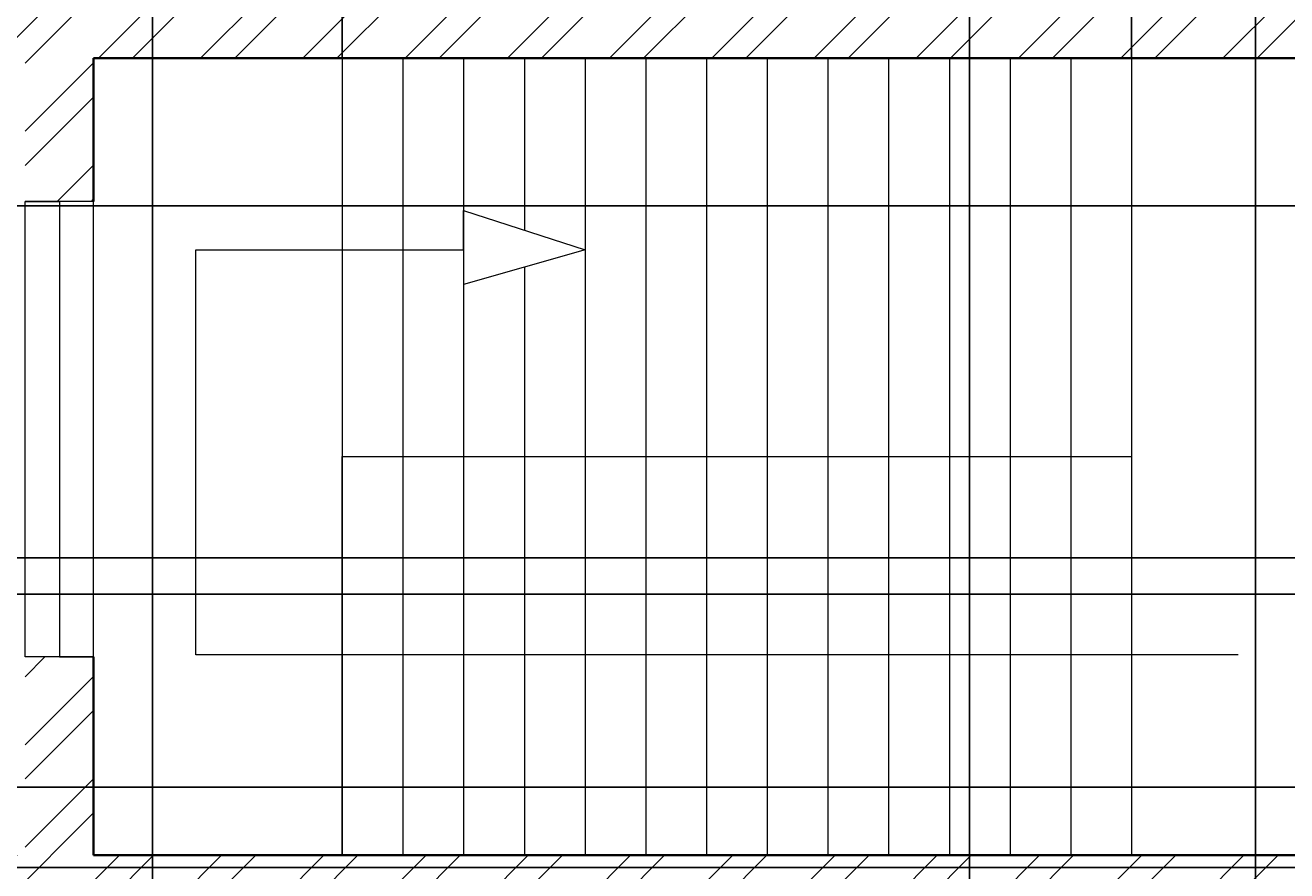
# Model space of a CAD drawing. Units: inches. Extents: x 1601 to 2297, y 1496 to 2631.
# Tile 14 of 57: x 1723 to 1889, y 2029 to 2141. Entities that reach past the tile are written whole.
import ezdxf

# ---------------------------------------------------------------- set-up
doc = ezdxf.new("R2010")
doc.units = ezdxf.units.IN
for name, color, linetype, lineweight in [('A-ANNO-DIMS', 2, 'Continuous', 18), ('A-FLOR-STRS', 191, 'Continuous', 18), ('A-GLAZ', 161, 'Continuous', 20), ('A-WALL', 7, 'Continuous', 40), ('A-WALL-PATT', 215, 'Continuous', 13)]:
    doc.layers.add(name, color=color, linetype=linetype, lineweight=lineweight)
doc.styles.get("Standard").update_dxf_attribs({"font": 'arial.ttf'})
doc.dimstyles.get("Standard").update_dxf_attribs({"dimtxt": 0.18, "dimasz": 0.18, "dimexe": 0.18, "dimexo": 0.0625, "dimgap": 0.09, "dimtad": 0, "dimtih": 1, "dimtoh": 1, "dimdec": 4, "dimzin": 0, "dimdsep": 46, "dimtxsty": 'Standard', "dimcen": 0.09, "dimadec": 0, "dimazin": 0, "dimtfac": 1, "dimtdec": 4, "dimtofl": 0, "dimtmove": 0, "dimatfit": 3, "dimfxl": 1, "dimtolj": 1, "dimtzin": 0, "dimarcsym": 0})

# ---------------------------------------------------------------- blocks, each defined once
blk = doc.blocks.new('WIN-60IN-JAMB9')
for p, q in [((4.5, 60), (0, 60)), ((0, 60), (9, 60)), ((0, 60), (0, 0)), ((4.5, 0), (4.5, 60)), ((9, 60), (9, 0)), ((0, 0), (9, 0)), ((9, 0), (4.5, 0))]:
    blk.add_line(p, q)
blk = doc.blocks.new('*D33')
at = {"layer": 'A-ANNO-DIMS', "color": 0, "lineweight": -2, "transparency": 16777216}
for p, q in [((1764.34, 2136.39), (1764.34, 2581.06)), ((1764.52, 2580.88), (1816.06, 2580.88)), ((1868.16, 2580.88), (1816.62, 2580.88)), ((1868.34, 2136.39), (1868.34, 2581.06))]:
    blk.add_line(p, q, dxfattribs=at)
at = {"layer": 'A-ANNO-DIMS', "color": 0, "transparency": 16777216}
for points in [[(1764.52, 2580.91), (1764.52, 2580.85), (1764.34, 2580.88)], [(1868.16, 2580.91), (1868.16, 2580.85), (1868.34, 2580.88)]]:
    blk.add_solid(points, dxfattribs=at)
at = {"layer": 'Defpoints', "color": 0, "transparency": 16777216}
for p in [(1868.34, 2580.88), (1764.34, 2136.33), (1868.34, 2136.33)]:
    blk.add_point(p, dxfattribs=at)
at = {"layer": 'A-ANNO-DIMS', "color": 0, "transparency": 16777216, "insert": (1816.34, 2580.88), "char_height": 0.18, "attachment_point": 5}
blk.add_mtext('\\A1;104', dxfattribs=at)
blk = doc.blocks.new('*D36')
at = {"layer": 'A-ANNO-DIMS', "color": 0, "lineweight": -2, "transparency": 16777216}
for p, q in [((1686.04, 1635.39), (1686.04, 2581.06)), ((1686.22, 2580.88), (1712.36, 2580.88)), ((1739.15, 2580.88), (1713.01, 2580.88)), ((1739.33, 1635.39), (1739.33, 2581.06))]:
    blk.add_line(p, q, dxfattribs=at)
at = {"layer": 'A-ANNO-DIMS', "color": 0, "transparency": 16777216}
for points in [[(1686.22, 2580.91), (1686.22, 2580.85), (1686.04, 2580.88)], [(1739.15, 2580.91), (1739.15, 2580.85), (1739.33, 2580.88)]]:
    blk.add_solid(points, dxfattribs=at)
at = {"layer": 'Defpoints', "color": 0, "transparency": 16777216}
for p in [(1739.33, 2580.88), (1686.04, 1635.33), (1739.33, 1635.33)]:
    blk.add_point(p, dxfattribs=at)
at = {"layer": 'A-ANNO-DIMS', "color": 0, "transparency": 16777216, "insert": (1712.69, 2580.88), "char_height": 0.18, "attachment_point": 5}
blk.add_mtext('\\A1;53.3', dxfattribs=at)
blk = doc.blocks.new('*D42')
at = {"layer": 'A-ANNO-DIMS', "color": 0, "lineweight": -2, "transparency": 16777216}
for p, q in [((2177.97, 2065.7), (1637.31, 2065.7)), ((1637.49, 2065.52), (1637.49, 2047.88)), ((1637.49, 2029.88), (1637.49, 2047.51)), ((2177.97, 2029.7), (1637.31, 2029.7))]:
    blk.add_line(p, q, dxfattribs=at)
at = {"layer": 'A-ANNO-DIMS', "color": 0, "transparency": 16777216}
for points in [[(1637.46, 2065.52), (1637.52, 2065.52), (1637.49, 2065.7)], [(1637.46, 2029.88), (1637.52, 2029.88), (1637.49, 2029.7)]]:
    blk.add_solid(points, dxfattribs=at)
at = {"layer": 'Defpoints', "color": 0, "transparency": 16777216}
for p in [(1637.49, 2065.7), (2178.04, 2065.7), (2178.04, 2029.7)]:
    blk.add_point(p, dxfattribs=at)
at = {"layer": 'A-ANNO-DIMS', "color": 0, "transparency": 16777216, "insert": (1637.49, 2047.7), "char_height": 0.18, "attachment_point": 5}
blk.add_mtext('\\A1;36', dxfattribs=at)
blk = doc.blocks.new('*D44')
at = {"layer": 'A-ANNO-DIMS', "color": 0, "lineweight": -2, "transparency": 16777216}
for p, q in [((1958.97, 2116.84), (1637.31, 2116.84)), ((1637.49, 2116.66), (1637.49, 2093.85)), ((1637.49, 2070.67), (1637.49, 2093.48)), ((1958.97, 2070.49), (1637.31, 2070.49))]:
    blk.add_line(p, q, dxfattribs=at)
at = {"layer": 'A-ANNO-DIMS', "color": 0, "transparency": 16777216}
for points in [[(1637.46, 2116.66), (1637.52, 2116.66), (1637.49, 2116.84)], [(1637.46, 2070.67), (1637.52, 2070.67), (1637.49, 2070.49)]]:
    blk.add_solid(points, dxfattribs=at)
at = {"layer": 'Defpoints', "color": 0, "transparency": 16777216}
for p in [(1637.49, 2116.84), (1959.04, 2116.84), (1959.04, 2070.49)]:
    blk.add_point(p, dxfattribs=at)
at = {"layer": 'A-ANNO-DIMS', "color": 0, "transparency": 16777216, "insert": (1637.49, 2093.67), "char_height": 0.18, "attachment_point": 5}
blk.add_mtext('\\A1;46.34', dxfattribs=at)
blk = doc.blocks.new('*D45')
at = {"layer": 'A-ANNO-DIMS', "color": 0, "lineweight": -2, "transparency": 16777216}
for p, q in [((1958.97, 2040.3), (1637.31, 2040.3)), ((1637.49, 2040.12), (1637.49, 2024.57)), ((1637.49, 2008.66), (1637.49, 2024.21)), ((1958.97, 2008.48), (1637.31, 2008.48))]:
    blk.add_line(p, q, dxfattribs=at)
at = {"layer": 'A-ANNO-DIMS', "color": 0, "transparency": 16777216}
for points in [[(1637.46, 2040.12), (1637.52, 2040.12), (1637.49, 2040.3)], [(1637.46, 2008.66), (1637.52, 2008.66), (1637.49, 2008.48)]]:
    blk.add_solid(points, dxfattribs=at)
at = {"layer": 'Defpoints', "color": 0, "transparency": 16777216}
for p in [(1637.49, 2040.3), (1959.04, 2040.3), (1959.04, 2008.48)]:
    blk.add_point(p, dxfattribs=at)
at = {"layer": 'A-ANNO-DIMS', "color": 0, "transparency": 16777216, "insert": (1637.49, 2024.39), "char_height": 0.18, "attachment_point": 5}
blk.add_mtext('\\A1;31.83', dxfattribs=at)
blk = doc.blocks.new('*D46')
at = {"layer": 'A-ANNO-DIMS', "color": 0, "lineweight": -2, "transparency": 16777216}
for p, q in [((1846.99, 2347.76), (1846.99, 1513.75)), ((1884.68, 2347.76), (1884.68, 1513.75)), ((1847.17, 1513.93), (1865.44, 1513.93)), ((1884.5, 1513.93), (1866.23, 1513.93))]:
    blk.add_line(p, q, dxfattribs=at)
at = {"layer": 'A-ANNO-DIMS', "color": 0, "transparency": 16777216}
for points in [[(1847.17, 1513.96), (1847.17, 1513.9), (1846.99, 1513.93)], [(1884.5, 1513.96), (1884.5, 1513.9), (1884.68, 1513.93)]]:
    blk.add_solid(points, dxfattribs=at)
at = {"layer": 'Defpoints', "color": 0, "transparency": 16777216}
for p in [(1846.99, 2347.83), (1884.68, 2347.83), (1884.68, 1513.93)]:
    blk.add_point(p, dxfattribs=at)
at = {"layer": 'A-ANNO-DIMS', "color": 0, "transparency": 16777216, "insert": (1865.84, 1513.93), "char_height": 0.18, "attachment_point": 5}
blk.add_mtext('\\A1;37.68', dxfattribs=at)

msp = doc.modelspace()

# ---------------------------------------------------------------- hatches: boundary and pattern name
at = {"layer": 'A-WALL-PATT'}
h = msp.add_hatch(dxfattribs=at)
h.set_pattern_fill('ANSI32', color=256)
h.paths.add_polyline_path([(1973.9371, 2211.3254), (1893.0373, 2211.3254), (1893.0373, 2287.8254), (1884.6167, 2287.8254), (1884.6167, 2285.5754), (1884.6167, 2283.3254), (1888.5373, 2283.3254), (1888.5373, 2145.3254), (1695.0373, 2145.3254), (1695.0373, 2173.8724), (1690.5373, 2173.8724), (1686.0373, 2173.8724), (1686.0373, 2136.3254), (1722.5687, 2136.3254), (1722.5687, 2117.4352), (1731.5687, 2117.4352), (1731.5687, 2136.3254), (1893.0373, 2136.3254), (1893.0373, 2202.3254), (1959.0373, 2202.3254), (1959.0373, 2182.1303), (1968.0373, 2182.1303), (1968.0373, 2202.3254), (1973.9371, 2202.3254)])
h.paths.add_polyline_path([(2094.0373, 2274.6364), (2096.4294, 2274.6364), (2096.4294, 2276.8864), (2096.4294, 2279.1364), (2094.0373, 2279.1364), (2094.0373, 2290.8254), (2094.0373, 2295.3254), (2089.5373, 2295.3254), (2089.5373, 2230.8254), (2035.5373, 2230.8254), (2035.5373, 2299.8254), (2031.0373, 2299.8254), (2031.0373, 2211.3254), (2023.0065, 2211.3254), (2023.0065, 2202.3254), (2031.0373, 2202.3254), (2031.0373, 2140.8254), (1968.0373, 2140.8254), (1968.0373, 2145.9106), (1963.5373, 2145.9106), (1959.0373, 2145.9106), (1959.0373, 2116.839), (1963.5373, 2116.839), (1968.0373, 2116.839), (1968.0373, 2131.8254), (2031.0373, 2131.8254), (2031.0373, 2094.3254), (2031.0373, 2085.3254), (2031.0373, 2056.8254), (1968.0373, 2056.8254), (1968.0373, 2070.4947), (1963.5373, 2070.4947), (1959.0373, 2070.4947), (1959.0373, 2040.3029), (1968.0373, 2040.3029), (1968.0373, 2047.8254), (2031.0373, 2047.8254), (2031.0373, 1983.3254), (2031.0373, 1978.8254), (2021.1979, 1978.8254), (2021.1979, 1974.3254), (2031.0373, 1974.3254), (2031.0373, 1954.3528), (2035.5373, 1954.3528), (2035.5373, 1974.3254), (2035.5373, 1981.8254), (2055.5513, 1981.8254), (2055.5513, 1986.3254), (2035.5373, 1986.3254), (2035.5373, 2047.8254), (2040.0373, 2047.8254), (2040.0373, 2085.3254), (2040.0373, 2094.3254), (2040.0373, 2140.8254), (2035.5373, 2140.8254), (2035.5373, 2226.3254), (2089.5373, 2226.3254), (2094.0373, 2226.3254)])
h.paths.add_polyline_path([(2226.0373, 2230.8254), (2134.5373, 2230.8254), (2134.5373, 2233.5437), (2130.0373, 2233.5437), (2130.0373, 2226.3254), (2134.5373, 2226.3254), (2226.0373, 2226.3254)])
h.paths.add_polyline_path([(1807.1169, 1573.5395), (2055.0405, 1573.5395), (2055.0405, 1610.6322), (1807.1169, 1610.6322)], flags=9)
h.paths.add_polyline_path([(1841.1631, 1712.7967), (1870.3957, 1712.7967), (1870.3957, 1731.454), (1841.1631, 1731.454)], flags=9)
h.paths.add_polyline_path([(2144.3862, 1772.185), (2191.0233, 1772.185), (2191.0233, 1790.8423), (2144.3862, 1790.8423)], flags=9)
h.paths.add_polyline_path([(2143.0128, 1827.3312), (2177.9958, 1827.3312), (2177.9958, 1845.9886), (2143.0128, 1845.9886)], flags=9)
h.paths.add_polyline_path([(2041.2439, 1833.5691), (2070.8516, 1833.5691), (2070.8516, 1852.2264), (2041.2439, 1852.2264)], flags=9)
h.paths.add_polyline_path([(2097.2791, 1947.0598), (2134.2061, 1947.0598), (2134.2061, 1965.7171), (2097.2791, 1965.7171)], flags=9)
h.paths.add_polyline_path([(2214.995, 1904.3124), (2214.995, 1942.2899), (2196.3376, 1942.2899), (2196.3376, 1904.3124)], flags=9)
h.paths.add_polyline_path([(2186.6284, 2043.8031), (2219.7935, 2043.8031), (2219.7935, 2062.4605), (2186.6284, 2062.4605)], flags=9)
h.paths.add_polyline_path([(2064.0877, 2031.616), (2097.4949, 2031.616), (2097.4949, 2050.2734), (2064.0877, 2050.2734)], flags=9)
h.paths.add_polyline_path([(1973.1349, 1986.0688), (2008.4009, 1986.0688), (2008.4009, 2004.7261), (1973.1349, 2004.7261)], flags=25)
h.paths.add_polyline_path([(1976.3676, 2106.9635), (2005.7469, 2106.9635), (2005.7469, 2125.6209), (1976.3676, 2125.6209)], flags=25)
h.paths.add_polyline_path([(1991.7852, 2180.4863), (2027.0513, 2180.4863), (2027.0513, 2199.1437), (1991.7852, 2199.1437)], flags=25)
h.paths.add_polyline_path([(2106.1801, 2187.9359), (2152.2101, 2187.9359), (2152.2101, 2206.5932), (2106.1801, 2206.5932)], flags=9)
h.paths.add_polyline_path([(2148.6686, 2262.2542), (2182.318, 2262.2542), (2182.318, 2280.9115), (2148.6686, 2280.9115)], flags=9)
h.paths.add_polyline_path([(2041.6327, 2252.8147), (2071.2405, 2252.8147), (2071.2405, 2271.4721), (2041.6327, 2271.4721)], flags=25)
h.paths.add_polyline_path([(2063.9734, 2375.4265), (2100.9004, 2375.4265), (2100.9004, 2394.0839), (2063.9734, 2394.0839)], flags=9)
h.paths.add_polyline_path([(2216.4955, 2330.9748), (2216.4955, 2370.2654), (2197.8381, 2370.2654), (2197.8381, 2330.9748)], flags=9)
h.paths.add_polyline_path([(2179.1416, 2485.8687), (2212.3067, 2485.8687), (2212.3067, 2504.5261), (2179.1416, 2504.5261)], flags=9)
h.paths.add_polyline_path([(2078.7442, 2471.1516), (2112.1514, 2471.1516), (2112.1514, 2489.809), (2078.7442, 2489.809)], flags=9)
h.paths.add_polyline_path([(1915.9631, 2329.4668), (1952.8902, 2329.4668), (1952.8902, 2348.1241), (1915.9631, 2348.1241)], flags=9)
h.paths.add_polyline_path([(1904.3189, 2499.6709), (1940.4512, 2499.6709), (1940.4512, 2518.3282), (1904.3189, 2518.3282)], flags=9)
h.paths.add_polyline_path([(1892.3665, 2100.4595), (1925.6374, 2100.4595), (1925.6374, 2119.1169), (1892.3665, 2119.1169)], flags=9)
h.paths.add_polyline_path([(1909.2984, 1805.9631), (1946.2254, 1805.9631), (1946.2254, 1824.6205), (1909.2984, 1824.6205)], flags=9)
h.paths.add_polyline_path([(1934.6056, 1658.616), (1970.738, 1658.616), (1970.738, 1677.2733), (1934.6056, 1677.2733)], flags=9)
h.paths.add_polyline_path([(1711.2052, 1789.8902), (1750.0456, 1789.8902), (1750.0456, 1808.5476), (1711.2052, 1808.5476)], flags=9)
h.paths.add_polyline_path([(1742.7874, 1854.6743), (1771.9449, 1854.6743), (1771.9449, 1873.3317), (1742.7874, 1873.3317)], flags=9)
h.paths.add_polyline_path([(1807.3592, 1997.7912), (1850.1116, 1997.7912), (1850.1116, 2016.4486), (1807.3592, 2016.4486)], flags=9)
h.paths.add_polyline_path([(1717.4579, 2237.7844), (1760.2103, 2237.7844), (1760.2103, 2256.4417), (1717.4579, 2256.4417)], flags=25)
h.paths.add_polyline_path([(1780.9285, 2324.0623), (1810.086, 2324.0623), (1810.086, 2342.7197), (1780.9285, 2342.7197)], flags=9)
h.paths.add_polyline_path([(1837.696, 2449.2024), (1866.9286, 2449.2024), (1866.9286, 2467.8598), (1837.696, 2467.8598)], flags=9)
h.paths.add_polyline_path([(1712.7752, 2484.9404), (1751.6156, 2484.9404), (1751.6156, 2503.5977), (1712.7752, 2503.5977)], flags=9)
h = msp.add_hatch(dxfattribs=at)
h.set_pattern_fill('ANSI32', color=256)
h.paths.add_polyline_path([(2230.5373, 1861.8254), (2182.5373, 1861.8254), (2182.5373, 1885.3637), (2178.0373, 1885.3637), (2178.0373, 1861.8254), (2166.0373, 1861.8254), (2134.5373, 1861.8254), (2130.0373, 1861.8254), (2130.0373, 1841.4682), (2126.8833, 1841.4682), (2126.8833, 1836.9682), (2130.0373, 1836.9682), (2130.0373, 1822.7302), (2134.5373, 1822.7302), (2134.5373, 1857.3254), (2166.0373, 1857.3254), (2226.0373, 1857.3254), (2226.0373, 1846.1155), (2230.5373, 1846.1155)])
h.paths.add_polyline_path([(2226.0373, 1797.3254), (2134.5373, 1797.3254), (2134.5373, 1800.6636), (2132.2873, 1800.6636), (2130.0373, 1800.6636), (2130.0373, 1797.3254), (2130.0373, 1792.8254), (2167.7264, 1792.8254), (2226.0373, 1792.8254)])
h.paths.add_polyline_path([(2230.5373, 1822.1155), (2226.0373, 1822.1155), (2226.0373, 1760.8563), (2230.5373, 1760.8563)])
h.paths.add_polyline_path([(2230.5373, 1700.8563), (2226.0373, 1700.8563), (2226.0373, 1644.3254), (2140.2517, 1644.3254), (2140.2517, 1635.3254), (2230.5373, 1635.3254)])
h.paths.add_polyline_path([(2080.2517, 1639.8254), (2080.2517, 1644.3254), (2035.5373, 1644.3254), (2035.5373, 1792.8254), (2094.0373, 1792.8254), (2094.0373, 1797.3254), (2094.0373, 1836.9682), (2097.1057, 1836.9682), (2097.1057, 1839.2182), (2097.1057, 1841.4682), (2094.0373, 1841.4682), (2094.0373, 1862.2276), (2089.5373, 1862.2276), (2089.5373, 1797.3254), (2035.5373, 1797.3254), (2035.5373, 1857.3254), (2035.5373, 1885.0916), (2031.0373, 1885.0916), (2031.0373, 1710.3254), (2012.329, 1710.3254), (2012.329, 1701.3254), (2031.0373, 1701.3254), (2031.0373, 1644.3254), (2031.0373, 1635.3254), (2080.2517, 1635.3254)])
h.paths.add_polyline_path([(1836.0373, 1653.2033), (1842.6171, 1653.2033), (1842.6171, 1657.7033), (1842.6171, 1662.2033), (1831.5373, 1662.2033), (1831.5373, 1764.2033), (1835.3881, 1764.2033), (1835.3881, 1766.4533), (1835.3881, 1768.7033), (1831.5373, 1768.7033), (1827.0373, 1768.7033), (1827.0373, 1662.2033), (1827.0373, 1635.3254), (1836.0373, 1635.3254)])
h.paths.add_polyline_path([(1893.0373, 1701.3254), (1907.193, 1701.3254), (1907.193, 1705.8254), (1907.193, 1710.3254), (1893.0373, 1710.3254), (1893.0373, 1819.8254), (1882.6444, 1819.8254), (1882.6444, 1817.5754), (1882.6444, 1815.3254), (1888.5373, 1815.3254), (1888.5373, 1662.2033), (1884.0373, 1662.2033), (1866.6171, 1662.2033), (1866.6171, 1653.2033), (1882.391, 1653.2033), (1884.0373, 1653.2033), (1884.0373, 1635.3254), (1893.0373, 1635.3254)])
h.paths.add_polyline_path([(1739.3335, 1639.8254), (1739.3335, 1644.3254), (1695.0373, 1644.3254), (1695.0373, 1702.0135), (1690.5373, 1702.0135), (1686.0373, 1702.0135), (1686.0373, 1635.3254), (1739.3335, 1635.3254)])
h.paths.add_polyline_path([(1827.0373, 1644.3254), (1799.3335, 1644.3254), (1799.3335, 1635.3254), (1827.0373, 1635.3254)])
h.paths.add_polyline_path([(1695.0373, 1815.3254), (1849.2759, 1815.3254), (1849.2759, 1819.8254), (1807.5373, 1819.8254), (1807.5373, 1879.8254), (1851.1533, 1879.8254), (1851.1533, 1882.0754), (1851.1533, 1884.3254), (1799.3405, 1884.3254), (1799.3405, 1882.0754), (1799.3405, 1879.8254), (1803.0373, 1879.8254), (1803.0373, 1819.8254), (1695.0373, 1819.8254), (1695.0373, 1835.0458), (1690.5373, 1835.0458), (1686.0373, 1835.0458), (1686.0373, 1766.1753), (1695.0373, 1766.1753)])
h.paths.add_polyline_path([(1775.8157, 1884.3254), (1695.0373, 1884.3254), (1695.0373, 1912.9526), (1690.5373, 1912.9526), (1686.0373, 1912.9526), (1686.0373, 1859.0458), (1695.0373, 1859.0458), (1695.0373, 1879.8254), (1775.8157, 1879.8254)])
h.paths.add_polyline_path([(1893.0373, 2031.3254), (1731.5687, 2031.3254), (1731.5687, 2057.4352), (1722.5687, 2057.4352), (1722.5687, 2031.3254), (1686.0373, 2031.3254), (1686.0373, 1972.9526), (1695.0373, 1972.9526), (1695.0373, 2022.3254), (1888.5373, 2022.3254), (1888.5373, 1884.3254), (1883.4996, 1884.3254), (1883.4996, 1879.8254), (1893.0373, 1879.8254), (1893.0373, 1974.3254), (1976.6199, 1974.3254), (1976.6199, 1978.8254), (1968.0373, 1978.8254), (1968.0373, 1983.3254), (1968.0373, 2008.4756), (1963.5373, 2008.4756), (1959.0373, 2008.4756), (1959.0373, 1983.3254), (1893.0373, 1983.3254)])
h.paths.add_polyline_path([(2230.5373, 2140.4745), (2226.0373, 2140.4745), (2226.0373, 2094.3254), (2040.0373, 2094.3254), (2040.0373, 2085.3254), (2178.0373, 2085.3254), (2178.0373, 2065.6965), (2182.5373, 2065.6965), (2182.5373, 2085.3254), (2226.0373, 2085.3254), (2226.0373, 1986.3254), (2211.2679, 1986.3254), (2211.2679, 1981.8254), (2230.5373, 1981.8254)])
h.paths.add_polyline_path([(2187.6292, 1986.3254), (2182.5373, 1986.3254), (2182.5373, 2029.6965), (2178.0373, 2029.6965), (2178.0373, 1986.3254), (2099.05, 1986.3254), (2099.05, 1981.8254), (2178.0373, 1981.8254), (2178.0373, 1969.3637), (2182.5373, 1969.3637), (2182.5373, 1981.8254), (2187.6292, 1981.8254), (2187.6292, 1984.0754)])
h.paths.add_polyline_path([(1807.1169, 1573.5395), (2055.0405, 1573.5395), (2055.0405, 1610.6322), (1807.1169, 1610.6322)], flags=9)
h.paths.add_polyline_path([(1841.1631, 1712.7967), (1870.3957, 1712.7967), (1870.3957, 1731.454), (1841.1631, 1731.454)], flags=9)
h.paths.add_polyline_path([(2144.3862, 1772.185), (2191.0233, 1772.185), (2191.0233, 1790.8423), (2144.3862, 1790.8423)], flags=9)
h.paths.add_polyline_path([(2143.0128, 1827.3312), (2177.9958, 1827.3312), (2177.9958, 1845.9886), (2143.0128, 1845.9886)], flags=25)
h.paths.add_polyline_path([(2041.2439, 1833.5691), (2070.8516, 1833.5691), (2070.8516, 1852.2264), (2041.2439, 1852.2264)], flags=25)
h.paths.add_polyline_path([(2097.2791, 1947.0598), (2134.2061, 1947.0598), (2134.2061, 1965.7171), (2097.2791, 1965.7171)], flags=9)
h.paths.add_polyline_path([(2214.995, 1904.3124), (2214.995, 1942.2899), (2196.3376, 1942.2899), (2196.3376, 1904.3124)], flags=9)
h.paths.add_polyline_path([(2186.6284, 2043.8031), (2219.7935, 2043.8031), (2219.7935, 2062.4605), (2186.6284, 2062.4605)], flags=25)
h.paths.add_polyline_path([(2064.0877, 2031.616), (2097.4949, 2031.616), (2097.4949, 2050.2734), (2064.0877, 2050.2734)], flags=25)
h.paths.add_polyline_path([(1973.1349, 1986.0688), (2008.4009, 1986.0688), (2008.4009, 2004.7261), (1973.1349, 2004.7261)], flags=9)
h.paths.add_polyline_path([(1976.3676, 2106.9635), (2005.7469, 2106.9635), (2005.7469, 2125.6209), (1976.3676, 2125.6209)], flags=9)
h.paths.add_polyline_path([(1991.7852, 2180.4863), (2027.0513, 2180.4863), (2027.0513, 2199.1437), (1991.7852, 2199.1437)], flags=9)
h.paths.add_polyline_path([(2106.1801, 2187.9359), (2152.2101, 2187.9359), (2152.2101, 2206.5932), (2106.1801, 2206.5932)], flags=9)
h.paths.add_polyline_path([(2148.6686, 2262.2542), (2182.318, 2262.2542), (2182.318, 2280.9115), (2148.6686, 2280.9115)], flags=9)
h.paths.add_polyline_path([(2041.6327, 2252.8147), (2071.2405, 2252.8147), (2071.2405, 2271.4721), (2041.6327, 2271.4721)], flags=9)
h.paths.add_polyline_path([(2063.9734, 2375.4265), (2100.9004, 2375.4265), (2100.9004, 2394.0839), (2063.9734, 2394.0839)], flags=9)
h.paths.add_polyline_path([(2216.4955, 2330.9748), (2216.4955, 2370.2654), (2197.8381, 2370.2654), (2197.8381, 2330.9748)], flags=9)
h.paths.add_polyline_path([(2179.1416, 2485.8687), (2212.3067, 2485.8687), (2212.3067, 2504.5261), (2179.1416, 2504.5261)], flags=9)
h.paths.add_polyline_path([(2078.7442, 2471.1516), (2112.1514, 2471.1516), (2112.1514, 2489.809), (2078.7442, 2489.809)], flags=9)
h.paths.add_polyline_path([(1915.9631, 2329.4668), (1952.8902, 2329.4668), (1952.8902, 2348.1241), (1915.9631, 2348.1241)], flags=9)
h.paths.add_polyline_path([(1904.3189, 2499.6709), (1940.4512, 2499.6709), (1940.4512, 2518.3282), (1904.3189, 2518.3282)], flags=9)
h.paths.add_polyline_path([(1892.3665, 2100.4595), (1925.6374, 2100.4595), (1925.6374, 2119.1169), (1892.3665, 2119.1169)], flags=9)
h.paths.add_polyline_path([(1909.2984, 1805.9631), (1946.2254, 1805.9631), (1946.2254, 1824.6205), (1909.2984, 1824.6205)], flags=9)
h.paths.add_polyline_path([(1934.6056, 1658.616), (1970.738, 1658.616), (1970.738, 1677.2733), (1934.6056, 1677.2733)], flags=9)
h.paths.add_polyline_path([(1711.2052, 1789.8902), (1750.0456, 1789.8902), (1750.0456, 1808.5476), (1711.2052, 1808.5476)], flags=25)
h.paths.add_polyline_path([(1742.7874, 1854.6743), (1771.9449, 1854.6743), (1771.9449, 1873.3317), (1742.7874, 1873.3317)], flags=25)
h.paths.add_polyline_path([(1807.3592, 1997.7912), (1850.1116, 1997.7912), (1850.1116, 2016.4486), (1807.3592, 2016.4486)], flags=25)
h.paths.add_polyline_path([(1717.4579, 2237.7844), (1760.2103, 2237.7844), (1760.2103, 2256.4417), (1717.4579, 2256.4417)], flags=9)
h.paths.add_polyline_path([(1780.9285, 2324.0623), (1810.086, 2324.0623), (1810.086, 2342.7197), (1780.9285, 2342.7197)], flags=9)
h.paths.add_polyline_path([(1837.696, 2449.2024), (1866.9286, 2449.2024), (1866.9286, 2467.8598), (1837.696, 2467.8598)], flags=9)
h.paths.add_polyline_path([(1712.7752, 2484.9404), (1751.6156, 2484.9404), (1751.6156, 2503.5977), (1712.7752, 2503.5977)], flags=9)

# ---------------------------------------------------------------- linework, layer by layer
at = {"layer": 'A-FLOR-STRS'}
for p, q in [((1764.3371, 2136.3254), (1764.3371, 2031.3254)), ((1772.3371, 2136.3254), (1772.3371, 2031.3254)), ((1780.3371, 2136.3254), (1780.3371, 2031.3254)), ((1788.3371, 2136.3254), (1788.3371, 2113.6728)), ((1796.3371, 2136.3254), (1796.3371, 2031.3254)), ((1804.3371, 2136.3254), (1804.3371, 2031.3254)), ((1812.3371, 2136.3254), (1812.3371, 2031.3254)), ((1820.3371, 2136.3254), (1820.3371, 2031.3254)), ((1828.3371, 2136.3254), (1828.3371, 2031.3254)), ((1836.3371, 2136.3254), (1836.3371, 2031.3254)), ((1844.3371, 2136.3254), (1844.3371, 2031.3254)), ((1852.3371, 2136.3254), (1852.3371, 2031.3254)), ((1860.3371, 2136.3254), (1860.3371, 2031.3254)), ((1868.3371, 2136.3254), (1868.3371, 2031.3254)), ((1780.3371, 2111.0821), (1780.3371, 2116.2634)), ((1780.3371, 2116.2634), (1796.3371, 2111.0821)), ((1745.0425, 2057.7302), (1745.0425, 2111.0821)), ((1745.0425, 2111.0821), (1780.3371, 2111.0821)), ((1796.3371, 2111.0821), (1780.3371, 2106.5062)), ((1788.3371, 2108.7941), (1788.3371, 2031.3254)), ((1764.3371, 2031.3254), (1764.3371, 2083.8254)), ((1764.3371, 2083.8254), (1868.3371, 2083.8254)), ((1882.4099, 2057.7302), (1745.0425, 2057.7302))]:
    msp.add_line(p, q, dxfattribs=at)
at = {"layer": 'A-WALL'}
for p, q in [((1731.5687, 2136.3254), (1893.0373, 2136.3254)), ((1731.5687, 2117.4352), (1731.5687, 2136.3254)), ((1731.5687, 2031.3254), (1731.5687, 2057.4352)), ((1731.5687, 2031.3254), (1893.0373, 2031.3254))]:
    msp.add_line(p, q, dxfattribs=at)

# ---------------------------------------------------------------- block references
at = {"layer": 'A-GLAZ', "rotation": 180}
msp.add_blockref('WIN-60IN-JAMB9', (1731.569, 2117.4357), dxfattribs=at)

# ---------------------------------------------------------------- dimensions: what is measured, and where the dimension line sits
at = {"layer": 'A-ANNO-DIMS'}
for base, p1, p2, override, picture, middle in [((1739.3335, 2580.8754), (1686.0373, 1635.3254), (1739.3335, 1635.3254), {"dimdec": 1, "dimlfac": 1, "dimrnd": 0, "dimzin": 0, "dimdsep": 46, "dimlunit": 2}, '*D36', (1712.6854, 2580.8754)), ((1868.3371, 2580.8754), (1764.3371, 2136.3254), (1868.3371, 2136.3254), {"dimdec": 0, "dimlfac": 1, "dimrnd": 0, "dimzin": 0, "dimdsep": 46, "dimlunit": 2}, '*D33', (1816.3371, 2580.8754)), ((1884.6773, 1513.9279), (1846.9946, 2347.8254), (1884.6773, 2347.8254), {"dimdec": 2, "dimlfac": 1, "dimrnd": 0, "dimzin": 0, "dimdsep": 46, "dimlunit": 2}, '*D46', (1865.836, 1513.9279))]:
    dim = msp.add_linear_dim(base=base, p1=p1, p2=p2, dimstyle='Standard', override=override, dxfattribs=at)
    dim.commit()
    dim.dimension.update_dxf_attribs({"geometry": picture, "text_midpoint": middle})
for base, p1, p2, override, picture, middle in [((1637.4873, 2116.839), (1959.0373, 2070.4947), (1959.0373, 2116.839), {"dimdec": 2, "dimlfac": 1, "dimrnd": 0, "dimzin": 0, "dimdsep": 46, "dimlunit": 2}, '*D44', (1637.4873, 2093.6668)), ((1637.4873, 2065.6965), (2178.0373, 2029.6965), (2178.0373, 2065.6965), {"dimdec": 0, "dimlfac": 1, "dimrnd": 0, "dimzin": 0, "dimdsep": 46, "dimlunit": 2}, '*D42', (1637.4873, 2047.6965)), ((1637.4873, 2040.3029), (1959.0373, 2008.4756), (1959.0373, 2040.3029), {"dimdec": 2, "dimlfac": 1, "dimrnd": 0, "dimzin": 0, "dimdsep": 46, "dimlunit": 2}, '*D45', (1637.4873, 2024.3893))]:
    dim = msp.add_linear_dim(base=base, p1=p1, p2=p2, angle=90, dimstyle='Standard', override=override, dxfattribs=at)
    dim.commit()
    dim.dimension.update_dxf_attribs({"geometry": picture, "text_midpoint": middle})

doc.saveas('drawing.dxf')
